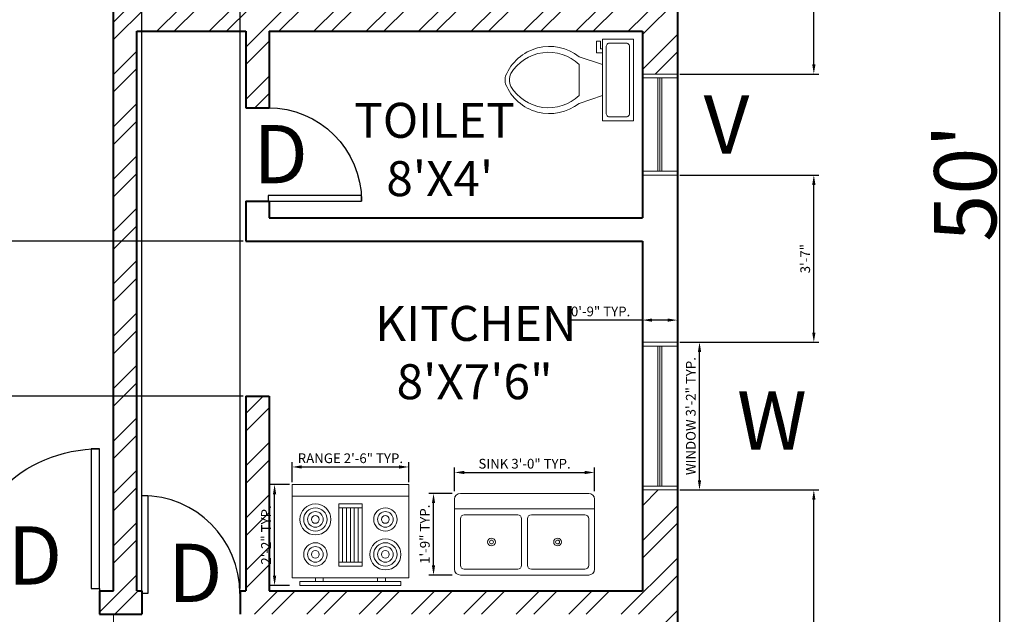
# Model space of a CAD drawing. Units: inches. Extents: x 1143 to 1626, y 7431 to 8140.
# Tile 3 of 4: x 1373 to 1626, y 7656 to 7809. Entities that reach past the tile are written whole.
import ezdxf

# ---------------------------------------------------------------- set-up
doc = ezdxf.new("R2010")
doc.units = ezdxf.units.IN
doc.linetypes.add('ACAD_ISO02W100', pattern=[15, 12, -3])
for name, color, linetype, lineweight in [('A-ANNO-DIMS', 4, 'Continuous', 18), ('A-DOOR', 3, 'Continuous', 25), ('A-FLOR-PRKG', 2, 'ACAD_ISO02W100', 18), ('A-GLAZ', 4, 'Continuous', 18), ('A-WALL', 2, 'Continuous', 40), ('A-WALL-PATT', 7, 'Continuous', 13)]:
    doc.layers.add(name, color=color, linetype=linetype, lineweight=lineweight)
for name, color, linetype, lineweight, true_color in [('A-ANNO-TEXT', 40, 'Continuous', 18, 0xf8d731), ('A-AREA-IDEN', 40, 'Continuous', 25, 0xf8d731), ('A-EQPM', 40, 'Continuous', 18, 0xf8d731), ('A-FLOR-FIXT', 40, 'Continuous', 18, 0xf8d731)]:
    doc.layers.add(name, color=color, linetype=linetype, lineweight=lineweight, true_color=true_color)
doc.styles.get("Standard").update_dxf_attribs({"font": 'arial.ttf'})
doc.dimstyles.new('ISO-25', dxfattribs={"dimtxt": 2.5, "dimasz": 2.5, "dimexe": 1.25, "dimexo": 0.625, "dimtad": 1, "dimdec": 0, "dimlunit": 3, "dimtxsty": 'Standard', "dimcen": 2.5, "dimadec": 0, "dimazin": 0, "dimtfac": 1, "dimtdec": 0, "dimtmove": 0, "dimatfit": 3, "dimfxl": 1, "dimarcsym": 0})

# ---------------------------------------------------------------- blocks, each defined once
blk = doc.blocks.new('*U8')
for p, q in [((0, 0), (0, -100)), ((750, 0), (750, -100))]:
    blk.add_line(p, q)
blk.add_lwpolyline([(0, 0), (0, 750), (43.75, 750), (43.75, 0)], close=True)
blk.add_arc((0, 0), 750, 0, 90)
blk = doc.blocks.new('Range-Oven - 30 in top')
for p, q in [((0, -3), (30, -3)), ((12, -6), (18, -6)), ((13, -20), (13, -6)), ((14, -6), (14, -20)), ((15, -20), (15, -6)), ((16, -6), (16, -20)), ((17, -20), (17, -6)), ((18, -20), (12, -20)), ((6, -24), (6, -25)), ((8, -25), (8, -24)), ((22, -25), (22, -24)), ((24, -24), (24, -25))]:
    blk.add_line(p, q)
for points in [[(0, -24), (0, 0), (30, 0), (30, -24)], [(12, -21), (12, -5), (18, -5), (18, -21)], [(2, -26), (2, -25), (28, -25), (28, -26)]]:
    blk.add_lwpolyline(points, close=True)
for centre, radius in [((6, -9), 4), ((6, -9), 3), ((6, -9), 2), ((24, -9), 3), ((24, -9), 2), ((6, -9), 1), ((24, -9), 1), ((6, -18), 3), ((24, -18), 4), ((24, -18), 3), ((6, -18), 2), ((6, -18), 1), ((24, -18), 2), ((24, -18), 1)]:
    blk.add_circle(centre, radius)
blk = doc.blocks.new('Sink-double - 36 in top')
for p, q in [((-18, -4), (18, -4)), ((-0.75, -18.5), (-0.75, -6.5)), ((0.75, -6.5), (0.75, -18.5))]:
    blk.add_line(p, q)
for points in [[(-16.5, 0), (16.5, 0)], [(-18, -19.5), (-18, -1.5)], [(18, -1.5), (18, -19.5)], [(-16.5, -18.5), (-16.5, -6.5)], [(-15.5, -5.5), (-1.75, -5.5)], [(1.75, -5.5), (15.5, -5.5)], [(16.5, -6.5), (16.5, -18.5)], [(-1.75, -19.5), (-15.5, -19.5)], [(15.5, -19.5), (1.75, -19.5)], [(16.5, -21), (-16.5, -21)]]:
    blk.add_lwpolyline(points)
for centre, radius in [((-8.5, -12.5), 1), ((-8.5, -12.5), 0.5), ((8.5, -12.5), 1), ((8.5, -12.5), 0.5)]:
    blk.add_circle(centre, radius)
for centre, radius, start, end in [((-16.5, -1.5), 1.5, 90, 180), ((16.5, -1.5), 1.5, 0, 90), ((-15.5, -6.5), 1, 90, 180), ((-1.75, -6.5), 1, 0, 90), ((1.75, -6.5), 1, 90, 180), ((15.5, -6.5), 1, 0, 90), ((-16.5, -19.5), 1.5, 180, 270), ((-15.5, -18.5), 1, 180, 270), ((-1.75, -18.5), 1, 270, 0), ((1.75, -18.5), 1, 180, 270), ((15.5, -18.5), 1, 270, 0), ((16.5, -19.5), 1.5, 270, 0)]:
    blk.add_arc(centre, radius, start, end)
blk = doc.blocks.new('Toilet - top')
for p, q in [((9.5, -6), (9.5, -2)), ((-10, -8.5), (-8, -8.5)), ((-10, -9.5), (-10, -8.5)), ((-7, -9.5), (-10, -9.5)), ((-8, -8.5), (-8, -8)), ((-7, -8), (-7, -9.5)), ((-4, -8), (-6, -14)), ((4, -8), (6, -14)), ((4, -14), (-4, -14))]:
    blk.add_line(p, q)
blk.add_lwpolyline([(10.5, -8), (10.5, 0), (-10.5, 0), (-10.5, -8)], close=True)
for points in [[(-9.5, -2), (-9.5, -6)], [(8.5, -1), (-8.5, -1)], [(-8.5, -7), (8.5, -7)]]:
    blk.add_lwpolyline(points)
for centre, radius, start, end in [((-8.62, -1.88), 0.884, 81.8699, 188.1301), ((8.62, -1.88), 0.884, 351.8699, 98.1301), ((-8.62, -6.12), 0.884, 171.8699, 278.1301), ((8.62, -6.12), 0.884, 261.8699, 8.1301), ((3.52, -21.58), 12.17, 141.4691, 247.9714), ((4.2, -21.82), 11.33, 136.3677, 238.9468), ((-3.52, -21.58), 12.17, 292.0284, 38.5307), ((-4.2, -21.82), 11.33, 301.053, 43.6321), ((0, -27.88), 4, 245.7318, 294.2682), ((0, -29), 4, 254.8605, 285.1395)]:
    blk.add_arc(centre, radius, start, end)
blk = doc.blocks.new('*D59')
at = {"layer": 'A-ANNO-DIMS', "color": 0, "lineweight": -2, "transparency": 16777216}
for p, q in [((1542.48, 8067.4), (1625.93, 8067.4)), ((1624.68, 8064.9), (1624.68, 7469.9)), ((1542.48, 7467.4), (1625.93, 7467.4))]:
    blk.add_line(p, q, dxfattribs=at)
at = {"layer": 'A-ANNO-DIMS', "color": 0, "transparency": 16777216}
for points in [[(1624.27, 8064.9), (1625.1, 8064.9), (1624.68, 8067.4)], [(1624.27, 7469.9), (1625.1, 7469.9), (1624.68, 7467.4)]]:
    blk.add_solid(points, dxfattribs=at)
at = {"layer": 'Defpoints', "color": 0, "transparency": 16777216}
for p in [(1541.85, 8067.4), (1541.85, 7467.4), (1624.68, 7467.4)]:
    blk.add_point(p, dxfattribs=at)
at = {"layer": 'A-ANNO-DIMS', "color": 0, "transparency": 16777216, "insert": (1615.89, 7767.4), "char_height": 2.5, "attachment_point": 5, "rotation": 90}
blk.add_mtext("{\\H6.4x;50'}", dxfattribs=at)
blk = doc.blocks.new('WIN-36IN')
for p, q in [((0, 9), (0, 0)), ((1, 9), (1, 0)), ((37, 9), (37, 0)), ((38, 9), (38, 0)), ((1, 5), (37, 5)), ((1, 4.5), (37, 4.5)), ((1, 4), (37, 4))]:
    blk.add_line(p, q)
blk = doc.blocks.new('WIN-24IN')
for p, q in [((0, 9), (0, 0)), ((1, 9), (1, 0)), ((25, 9), (25, 0)), ((26, 9), (26, 0)), ((1, 5), (25, 5)), ((1, 4.5), (25, 4.5)), ((1, 4), (25, 4))]:
    blk.add_line(p, q)
blk = doc.blocks.new('*D62')
at = {"layer": 'A-ANNO-DIMS', "color": 0, "lineweight": -2, "transparency": 16777216}
for p, q in [((1542.48, 7726.4), (1548.8, 7726.4)), ((1547.55, 7690.9), (1547.55, 7723.9)), ((1542.48, 7688.4), (1548.8, 7688.4))]:
    blk.add_line(p, q, dxfattribs=at)
at = {"layer": 'A-ANNO-DIMS', "color": 0, "transparency": 16777216}
for points in [[(1547.13, 7723.9), (1547.97, 7723.9), (1547.55, 7726.4)], [(1547.13, 7690.9), (1547.97, 7690.9), (1547.55, 7688.4)]]:
    blk.add_solid(points, dxfattribs=at)
at = {"layer": 'Defpoints', "color": 0, "transparency": 16777216}
for p in [(1541.85, 7726.4), (1547.55, 7726.4), (1541.85, 7688.4)]:
    blk.add_point(p, dxfattribs=at)
at = {"layer": 'A-ANNO-DIMS', "color": 0, "transparency": 16777216, "insert": (1545.63, 7707.4), "char_height": 2.5, "attachment_point": 5, "rotation": 90}
blk.add_mtext('WINDOW 3\'-2" TYP.', dxfattribs=at)
blk = doc.blocks.new('*D63')
at = {"layer": 'A-ANNO-DIMS', "color": 0, "lineweight": -2, "transparency": 16777216}
for p, q in [((1532.85, 7727.02), (1532.85, 7733.35)), ((1541.85, 7727.02), (1541.85, 7733.35)), ((1532.85, 7732.1), (1513.86, 7732.1)), ((1539.35, 7732.1), (1535.35, 7732.1))]:
    blk.add_line(p, q, dxfattribs=at)
at = {"layer": 'A-ANNO-DIMS', "color": 0, "transparency": 16777216}
for points in [[(1535.35, 7732.51), (1535.35, 7731.68), (1532.85, 7732.1)], [(1539.35, 7732.51), (1539.35, 7731.68), (1541.85, 7732.1)]]:
    blk.add_solid(points, dxfattribs=at)
at = {"layer": 'Defpoints', "color": 0, "transparency": 16777216}
for p in [(1532.85, 7732.1), (1532.85, 7726.4), (1541.85, 7726.4)]:
    blk.add_point(p, dxfattribs=at)
at = {"layer": 'A-ANNO-DIMS', "color": 0, "transparency": 16777216, "insert": (1522.11, 7734), "char_height": 2.5, "attachment_point": 5}
blk.add_mtext('0\'-9" TYP.', dxfattribs=at)
blk = doc.blocks.new('*D76')
at = {"layer": 'A-ANNO-DIMS', "color": 0, "lineweight": -2, "transparency": 16777216}
for p, q in [((1442.77, 7690.44), (1442.77, 7695.56)), ((1472.77, 7690.44), (1472.77, 7695.56)), ((1445.27, 7694.31), (1470.27, 7694.31))]:
    blk.add_line(p, q, dxfattribs=at)
at = {"layer": 'A-ANNO-DIMS', "color": 0, "transparency": 16777216}
for points in [[(1445.27, 7694.73), (1445.27, 7693.89), (1442.77, 7694.31)], [(1470.27, 7694.73), (1470.27, 7693.89), (1472.77, 7694.31)]]:
    blk.add_solid(points, dxfattribs=at)
at = {"layer": 'Defpoints', "color": 0, "transparency": 16777216}
for p in [(1472.77, 7694.31), (1442.77, 7689.81), (1472.77, 7689.81)]:
    blk.add_point(p, dxfattribs=at)
at = {"layer": 'A-ANNO-DIMS', "color": 0, "transparency": 16777216, "insert": (1457.77, 7696.23), "char_height": 2.5, "attachment_point": 5}
blk.add_mtext('RANGE 2\'-6" TYP.', dxfattribs=at)
blk = doc.blocks.new('*D77')
at = {"layer": 'A-ANNO-DIMS', "color": 0, "lineweight": -2, "transparency": 16777216}
for p, q in [((1442.15, 7689.81), (1437.02, 7689.81)), ((1438.27, 7666.31), (1438.27, 7687.31)), ((1442.15, 7663.81), (1437.02, 7663.81))]:
    blk.add_line(p, q, dxfattribs=at)
at = {"layer": 'A-ANNO-DIMS', "color": 0, "transparency": 16777216}
for points in [[(1437.86, 7687.31), (1438.69, 7687.31), (1438.27, 7689.81)], [(1437.86, 7666.31), (1438.69, 7666.31), (1438.27, 7663.81)]]:
    blk.add_solid(points, dxfattribs=at)
at = {"layer": 'Defpoints', "color": 0, "transparency": 16777216}
for p in [(1438.27, 7689.81), (1442.77, 7689.81), (1442.77, 7663.81)]:
    blk.add_point(p, dxfattribs=at)
at = {"layer": 'A-ANNO-DIMS', "color": 0, "transparency": 16777216, "insert": (1436.39, 7676.81), "char_height": 2.5, "attachment_point": 5, "rotation": 90}
blk.add_mtext('2\'-2" TYP.', dxfattribs=at)
blk = doc.blocks.new('*D78')
at = {"layer": 'A-ANNO-DIMS', "color": 0, "lineweight": -2, "transparency": 16777216}
for p, q in [((1484.55, 7688.12), (1484.55, 7694.15)), ((1487.05, 7692.9), (1518.05, 7692.9)), ((1520.55, 7688.12), (1520.55, 7694.15))]:
    blk.add_line(p, q, dxfattribs=at)
at = {"layer": 'A-ANNO-DIMS', "color": 0, "transparency": 16777216}
for points in [[(1487.05, 7693.31), (1487.05, 7692.48), (1484.55, 7692.9)], [(1518.05, 7693.31), (1518.05, 7692.48), (1520.55, 7692.9)]]:
    blk.add_solid(points, dxfattribs=at)
at = {"layer": 'Defpoints', "color": 0, "transparency": 16777216}
for p in [(1520.55, 7692.9), (1484.55, 7687.5), (1520.55, 7687.5)]:
    blk.add_point(p, dxfattribs=at)
at = {"layer": 'A-ANNO-DIMS', "color": 0, "transparency": 16777216, "insert": (1502.55, 7694.82), "char_height": 2.5, "attachment_point": 5}
blk.add_mtext('SINK 3\'-0" TYP.', dxfattribs=at)
blk = doc.blocks.new('*D79')
at = {"layer": 'A-ANNO-DIMS', "color": 0, "lineweight": -2, "transparency": 16777216}
for p, q in [((1483.92, 7687.5), (1477.9, 7687.5)), ((1479.15, 7669), (1479.15, 7685)), ((1483.92, 7666.5), (1477.9, 7666.5))]:
    blk.add_line(p, q, dxfattribs=at)
at = {"layer": 'A-ANNO-DIMS', "color": 0, "transparency": 16777216}
for points in [[(1478.73, 7685), (1479.56, 7685), (1479.15, 7687.5)], [(1478.73, 7669), (1479.56, 7669), (1479.15, 7666.5)]]:
    blk.add_solid(points, dxfattribs=at)
at = {"layer": 'Defpoints', "color": 0, "transparency": 16777216}
for p in [(1479.15, 7687.5), (1484.55, 7687.5), (1484.55, 7666.5)]:
    blk.add_point(p, dxfattribs=at)
at = {"layer": 'A-ANNO-DIMS', "color": 0, "transparency": 16777216, "insert": (1477.24, 7677), "char_height": 2.5, "attachment_point": 5, "rotation": 90}
blk.add_mtext('1\'-9" TYP.', dxfattribs=at)
blk = doc.blocks.new('*D94')
at = {"layer": 'A-ANNO-DIMS', "color": 0, "lineweight": -2, "transparency": 16777216}
for p, q in [((1542.48, 7688.4), (1578.2, 7688.4)), ((1576.95, 7469.9), (1576.95, 7685.9)), ((1542.48, 7467.4), (1578.2, 7467.4))]:
    blk.add_line(p, q, dxfattribs=at)
at = {"layer": 'A-ANNO-DIMS', "color": 0, "transparency": 16777216}
for points in [[(1576.53, 7685.9), (1577.37, 7685.9), (1576.95, 7688.4)], [(1576.53, 7469.9), (1577.37, 7469.9), (1576.95, 7467.4)]]:
    blk.add_solid(points, dxfattribs=at)
at = {"layer": 'Defpoints', "color": 0, "transparency": 16777216}
for p in [(1541.85, 7688.4), (1576.95, 7688.4), (1541.85, 7467.4)]:
    blk.add_point(p, dxfattribs=at)
at = {"layer": 'A-ANNO-DIMS', "color": 0, "transparency": 16777216, "insert": (1575.05, 7577.9), "char_height": 2.5, "attachment_point": 5, "rotation": 90}
blk.add_mtext('18\'-5"', dxfattribs=at)
blk = doc.blocks.new('*D95')
at = {"layer": 'A-ANNO-DIMS', "color": 0, "lineweight": -2, "transparency": 16777216}
for p, q in [((1542.48, 7769.4), (1578.2, 7769.4)), ((1576.95, 7728.9), (1576.95, 7766.9)), ((1542.48, 7726.4), (1578.2, 7726.4))]:
    blk.add_line(p, q, dxfattribs=at)
at = {"layer": 'A-ANNO-DIMS', "color": 0, "transparency": 16777216}
for points in [[(1576.53, 7766.9), (1577.37, 7766.9), (1576.95, 7769.4)], [(1576.53, 7728.9), (1577.37, 7728.9), (1576.95, 7726.4)]]:
    blk.add_solid(points, dxfattribs=at)
at = {"layer": 'Defpoints', "color": 0, "transparency": 16777216}
for p in [(1541.85, 7769.4), (1576.95, 7769.4), (1541.85, 7726.4)]:
    blk.add_point(p, dxfattribs=at)
at = {"layer": 'A-ANNO-DIMS', "color": 0, "transparency": 16777216, "insert": (1575.05, 7747.9), "char_height": 2.5, "attachment_point": 5, "rotation": 90}
blk.add_mtext('3\'-7"', dxfattribs=at)
blk = doc.blocks.new('*D96')
at = {"layer": 'A-ANNO-DIMS', "color": 0, "lineweight": -2, "transparency": 16777216}
for p, q in [((1542.48, 7853.4), (1578.2, 7853.4)), ((1576.95, 7797.9), (1576.95, 7850.9)), ((1542.48, 7795.4), (1578.2, 7795.4))]:
    blk.add_line(p, q, dxfattribs=at)
at = {"layer": 'A-ANNO-DIMS', "color": 0, "transparency": 16777216}
for points in [[(1576.53, 7850.9), (1577.37, 7850.9), (1576.95, 7853.4)], [(1576.53, 7797.9), (1577.37, 7797.9), (1576.95, 7795.4)]]:
    blk.add_solid(points, dxfattribs=at)
at = {"layer": 'Defpoints', "color": 0, "transparency": 16777216}
for p in [(1541.85, 7853.4), (1576.95, 7853.4), (1541.85, 7795.4)]:
    blk.add_point(p, dxfattribs=at)
at = {"layer": 'A-ANNO-DIMS', "color": 0, "transparency": 16777216, "insert": (1575.05, 7824.4), "char_height": 2.5, "attachment_point": 5, "rotation": 90}
blk.add_mtext('4\'-10"', dxfattribs=at)
blk = doc.blocks.new('*D102')
at = {"layer": 'A-ANNO-DIMS', "color": 0, "lineweight": -2, "transparency": 16777216}
for p, q in [((1404.17, 7663.02), (1404.17, 8103.75)), ((1429.38, 7663.02), (1429.38, 8103.75)), ((1406.67, 8102.5), (1426.88, 8102.5))]:
    blk.add_line(p, q, dxfattribs=at)
at = {"layer": 'A-ANNO-DIMS', "color": 0, "transparency": 16777216}
for points in [[(1406.67, 8102.91), (1406.67, 8102.08), (1404.17, 8102.5)], [(1426.88, 8102.91), (1426.88, 8102.08), (1429.38, 8102.5)]]:
    blk.add_solid(points, dxfattribs=at)
at = {"layer": 'Defpoints', "color": 0, "transparency": 16777216}
for p in [(1429.38, 8102.5), (1404.17, 7662.4), (1429.38, 7662.4)]:
    blk.add_point(p, dxfattribs=at)
at = {"layer": 'A-ANNO-DIMS', "color": 0, "transparency": 16777216, "insert": (1416.78, 8104.38), "char_height": 2.5, "attachment_point": 5}
blk.add_mtext('2\'-1"', dxfattribs=at)
blk = doc.blocks.new('*D103')
at = {"layer": 'A-ANNO-DIMS', "color": 0, "lineweight": -2, "transparency": 16777216}
for p, q in [((1430.23, 7752.4), (1145.5, 7752.4)), ((1146.75, 7715.06), (1146.75, 7749.9)), ((1430.23, 7712.56), (1145.5, 7712.56))]:
    blk.add_line(p, q, dxfattribs=at)
at = {"layer": 'A-ANNO-DIMS', "color": 0, "transparency": 16777216}
for points in [[(1146.33, 7749.9), (1147.17, 7749.9), (1146.75, 7752.4)], [(1146.33, 7715.06), (1147.17, 7715.06), (1146.75, 7712.56)]]:
    blk.add_solid(points, dxfattribs=at)
at = {"layer": 'Defpoints', "color": 0, "transparency": 16777216}
for p in [(1146.75, 7752.4), (1430.85, 7752.4), (1430.85, 7712.56)]:
    blk.add_point(p, dxfattribs=at)
at = {"layer": 'A-ANNO-DIMS', "color": 0, "transparency": 16777216, "insert": (1144.85, 7732.48), "char_height": 2.5, "attachment_point": 5, "rotation": 90}
blk.add_mtext('3\'-4"', dxfattribs=at)

msp = doc.modelspace()

# ---------------------------------------------------------------- hatches: boundary and pattern name
at = {"layer": 'A-WALL-PATT'}
h = msp.add_hatch(dxfattribs=at)
h.set_pattern_fill('ANSI32', color=256)
h.paths.add_polyline_path([(1240.85, 8067.4), (1181.85, 8067.4), (1181.85, 8017.4), (1190.85, 8017.4), (1190.85, 8058.4), (1240.85, 8058.4)])
h.paths.add_polyline_path([(1541.85, 8067.4), (1486.85, 8067.4), (1486.85, 8058.4), (1532.85, 8058.4), (1532.85, 8017.4), (1541.85, 8017.4)], flags=17)
h.paths.add_polyline_path([(1352.85, 8067.4), (1278.85, 8067.4), (1278.85, 8058.4), (1328.85, 8058.4), (1328.85, 7938.4), (1319.96, 7938.4), (1319.96, 7932.4), (1334.85, 7932.4), (1334.85, 7956.4), (1338.11, 7956.4), (1338.11, 7962.4), (1334.85, 7962.4), (1334.85, 8010.4), (1396.85, 8010.4), (1396.85, 7962.4), (1386.11, 7962.4), (1386.11, 7956.4), (1396.85, 7956.4), (1396.85, 7662.4), (1393.24, 7662.4), (1393.24, 7656.4), (1404.17, 7656.4), (1404.17, 7662.4), (1402.85, 7662.4), (1402.85, 7806.4), (1430.85, 7806.4), (1430.85, 7786.73), (1436.85, 7786.73), (1436.85, 7806.4), (1532.85, 7806.4), (1532.85, 7795.4), (1541.85, 7795.4), (1541.85, 7853.4), (1532.85, 7853.4), (1532.85, 7812.4), (1402.85, 7812.4), (1402.85, 7932.4), (1419.12, 7932.4), (1419.12, 7938.4), (1402.85, 7938.4), (1402.85, 8058.4), (1448.85, 8058.4), (1448.85, 8067.4), (1378.85, 8067.4), (1378.85, 8058.4), (1396.85, 8058.4), (1396.85, 8016.4), (1334.85, 8016.4), (1334.85, 8058.4), (1352.85, 8058.4)])
h.paths.add_polyline_path([(1283.96, 7938.4), (1190.85, 7938.4), (1190.85, 7979.4), (1181.85, 7979.4), (1181.85, 7903.4), (1190.85, 7903.4), (1190.85, 7932.4), (1238.85, 7932.4), (1238.85, 7848.4), (1234.31, 7848.4), (1234.31, 7842.4), (1244.85, 7842.4), (1244.85, 7932.4), (1283.96, 7932.4)])
h.paths.add_polyline_path([(1541.85, 7979.4), (1532.85, 7979.4), (1532.85, 7938.4), (1455.12, 7938.4), (1455.12, 7932.4), (1532.85, 7932.4), (1532.85, 7891.4), (1541.85, 7891.4)], flags=17)
h.paths.add_polyline_path([(1210.81, 7716.4), (1190.85, 7716.4), (1190.85, 7745.4), (1181.85, 7745.4), (1181.85, 7663.4), (1190.85, 7663.4), (1190.85, 7710.4), (1210.81, 7710.4)])
h.paths.add_polyline_path([(1232.89, 7871.85), (1232.89, 7871.89), (1234.29, 7871.89), (1234.29, 7847.89), (1232.89, 7847.89), (1232.89, 7871.85, 0.385662), (1210.31, 7848.85), (1210.31, 7842.4), (1190.85, 7842.4), (1190.85, 7806.4), (1244.85, 7806.4), (1244.85, 7716.4), (1325.66, 7716.4), (1334.85, 7716.4), (1334.85, 7706.63), (1328.13, 7706.63), (1328.13, 7704.53), (1292.13, 7704.53), (1292.13, 7706.63), (1328.85, 7706.63), (1328.85, 7710.4), (1325.66, 7710.4), (1234.81, 7710.4), (1234.81, 7716.6), (1233.41, 7716.6), (1233.41, 7740.6), (1234.81, 7740.6), (1234.81, 7716.4), (1238.85, 7716.4), (1238.85, 7800.4), (1190.85, 7800.4), (1190.85, 7770.4), (1186.85, 7770.4), (1186.85, 7746.4), (1185.85, 7746.4), (1185.85, 7770.4), (1181.85, 7770.4), (1181.85, 7878.4), (1190.85, 7878.4), (1190.85, 7848.4), (1210.3, 7848.4, -0.391105)])
h.paths.add_polyline_path([(1541.85, 7688.4), (1532.85, 7688.4), (1532.85, 7662.4), (1436.85, 7662.4), (1436.85, 7712.56), (1430.85, 7712.56), (1430.85, 7662.4), (1429.38, 7656.4), (1532.85, 7656.4), (1532.85, 7467.4), (1541.85, 7467.4)])
h.paths.add_polyline_path([(1334.85, 7656.4), (1357.24, 7656.4), (1357.24, 7662.4), (1334.85, 7662.4), (1334.85, 7670.63), (1328.85, 7670.63), (1328.85, 7618.14), (1334.85, 7618.14)])
h.paths.add_polyline_path([(1190.85, 7572.4), (1334.85, 7572.4), (1334.85, 7582.14), (1328.85, 7582.14), (1328.85, 7578.4), (1190.85, 7578.4), (1190.85, 7625.4), (1181.85, 7625.4), (1181.85, 7467.4), (1324.72, 7467.4), (1324.72, 7476.4), (1190.85, 7476.4)])

# ---------------------------------------------------------------- linework, layer by layer
at = {"layer": 'A-FLOR-PRKG'}
msp.add_line((1396.85, 7656.4), (1396.85, 7476.4), dxfattribs=at)
at = {"layer": 'A-WALL'}
for p, q in [((1541.85, 8067.4), (1541.85, 7467.4)), ((1396.85, 7662.4), (1396.85, 7956.4)), ((1402.85, 7806.4), (1430.85, 7806.4)), ((1402.85, 7662.4), (1402.85, 7806.4)), ((1430.85, 7806.4), (1430.85, 7786.73)), ((1436.85, 7806.4), (1436.85, 7786.73)), ((1436.85, 7806.4), (1532.85, 7806.4)), ((1532.85, 7806.4), (1532.85, 7758.4)), ((1430.85, 7786.73), (1436.85, 7786.73)), ((1430.85, 7762.73), (1436.85, 7762.73)), ((1430.85, 7762.73), (1430.85, 7752.4)), ((1436.85, 7762.73), (1436.85, 7758.4)), ((1436.85, 7758.4), (1532.85, 7758.4)), ((1430.85, 7752.4), (1532.85, 7752.4)), ((1532.85, 7752.4), (1532.85, 7662.4)), ((1430.85, 7712.56), (1436.85, 7712.56)), ((1430.85, 7712.56), (1430.85, 7662.4)), ((1436.85, 7712.56), (1436.85, 7662.4)), ((1393.24, 7662.4), (1393.24, 7656.4)), ((1393.24, 7662.4), (1396.85, 7662.4)), ((1402.85, 7662.4), (1404.17, 7662.4)), ((1404.17, 7662.4), (1404.17, 7656.4)), ((1429.38, 7662.4), (1429.38, 7656.4)), ((1429.38, 7662.4), (1430.85, 7662.4)), ((1436.85, 7662.4), (1532.85, 7662.4)), ((1393.24, 7656.4), (1404.17, 7656.4))]:
    msp.add_line(p, q, dxfattribs=at)

# ---------------------------------------------------------------- block references
at = {"layer": 'A-DOOR', "xscale": -0.0320363486803998, "yscale": 0.0320363486803998, "zscale": 0.0320363486803998, "rotation": 270}
msp.add_blockref('*U8', (1436.6, 7762.73), dxfattribs=at)
at = {"layer": 'A-DOOR'}
for p, xscale, yscale, zscale in [((1393.24, 7663), -0.0480000000000001, 0.0480000000000001, 0.0480000000000001), ((1404.17, 7661.75), 0.0336011074731409, 0.0336011074731409, 0.0336011074731409)]:
    msp.add_blockref('*U8', p, dxfattribs=dict(at, xscale=xscale, yscale=yscale, zscale=zscale))
at = {"layer": 'A-EQPM'}
msp.add_blockref('Range-Oven - 30 in top', (1442.77, 7689.81), dxfattribs=at)
at = {"layer": 'A-FLOR-FIXT', "rotation": 270}
msp.add_blockref('Toilet - top', (1530.56, 7793.87), dxfattribs=at)
at = {"layer": 'A-FLOR-FIXT'}
msp.add_blockref('Sink-double - 36 in top', (1502.55, 7687.5), dxfattribs=at)
at = {"layer": 'A-GLAZ'}
for name, p, rotation in [('WIN-24IN', (1532.85, 7795.4), 269.9999999999985), ('WIN-36IN', (1541.85, 7688.4), 89.99999999999628)]:
    msp.add_blockref(name, p, dxfattribs=dict(at, rotation=rotation))

# ---------------------------------------------------------------- texts
at = {"layer": 'A-ANNO-TEXT', "char_height": 15, "attachment_point": 1}
for s, insert in [('{V}', (1548.6, 7789.96)), ('{D}', (1432.77, 7782.3)), ('{W}', (1557.19, 7713.76)), ('{D}', (1369.59, 7679.04)), ('{D}', (1410.82, 7674.56))]:
    msp.add_mtext_dynamic_manual_height_columns(s, width=1087.9578, gutter_width=12.5, heights=[0], dxfattribs=dict(at, insert=insert))
at = {"layer": 'A-AREA-IDEN', "char_height": 9, "attachment_point": 1}
for s, insert in [("{       TOILET\\P          8'X4'}", (1439.5, 7788)), ('{     KITCHEN\\P       8\'X7\'6"}', (1450.4, 7735.75))]:
    msp.add_mtext_dynamic_manual_height_columns(s, width=1087.9578, gutter_width=12.5, heights=[0], dxfattribs=dict(at, insert=insert))

# ---------------------------------------------------------------- dimensions: what is measured, and where the dimension line sits
at = {"layer": 'A-ANNO-DIMS'}
dim = msp.add_linear_dim(base=(1429.38, 8102.5), p1=(1404.17, 7662.4), p2=(1429.38, 7662.4), dimstyle='ISO-25', override={"dimdec": 1, "dimlfac": 1, "dimrnd": 0, "dimzin": 1, "dimdsep": 46, "dimlunit": 4, "dimfrac": 2}, dxfattribs=at)
dim.commit()
dim.dimension.update_dxf_attribs({"geometry": '*D102', "text_midpoint": (1416.78, 8104.38)})
for base, p1, p2, angle, text, override, picture, middle in [((1624.68, 7467.4), (1541.85, 8067.4), (1541.85, 7467.4), 90, '{\\H6.4x;<>}', {"dimclrd": 0, "dimclre": 0, "dimclrt": 0}, '*D59', (1615.89, 7767.4)), ((1532.85, 7732.1), (1541.85, 7726.4), (1532.85, 7726.4), 180, '<> TYP.', {"dimdec": 1, "dimlfac": 1, "dimrnd": 0, "dimzin": 1, "dimdsep": 46, "dimlunit": 4, "dimfrac": 2}, '*D63', (1522.11, 7734)), ((1547.55, 7726.4), (1541.85, 7688.4), (1541.85, 7726.4), 90, 'WINDOW <> TYP.', {"dimdec": 1, "dimlfac": 1, "dimrnd": 0, "dimzin": 1, "dimdsep": 46, "dimlunit": 4, "dimfrac": 2}, '*D62', (1545.63, 7707.4)), ((1438.27, 7689.81), (1442.77, 7663.81), (1442.77, 7689.81), 90, '<> TYP.', {"dimdec": 1, "dimlfac": 1, "dimrnd": 0, "dimzin": 1, "dimdsep": 46, "dimlunit": 4, "dimfrac": 2}, '*D77', (1436.39, 7676.81)), ((1479.15, 7687.5), (1484.55, 7666.5), (1484.55, 7687.5), 90, '<> TYP.', {"dimdec": 1, "dimlfac": 1, "dimrnd": 0, "dimzin": 1, "dimdsep": 46, "dimlunit": 4, "dimfrac": 2}, '*D79', (1477.24, 7677))]:
    dim = msp.add_linear_dim(base=base, p1=p1, p2=p2, angle=angle, text=text, dimstyle='ISO-25', override=override, dxfattribs=at)
    dim.commit()
    dim.dimension.update_dxf_attribs({"geometry": picture, "text_midpoint": middle})
for base, p1, p2, picture, middle in [((1576.95, 7853.4), (1541.85, 7795.4), (1541.85, 7853.4), '*D96', (1575.05, 7824.4)), ((1576.95, 7769.4), (1541.85, 7726.4), (1541.85, 7769.4), '*D95', (1575.05, 7747.9)), ((1146.75, 7752.4), (1430.85, 7712.56), (1430.85, 7752.4), '*D103', (1144.85, 7732.48)), ((1576.95, 7688.4), (1541.85, 7467.4), (1541.85, 7688.4), '*D94', (1575.05, 7577.9))]:
    dim = msp.add_linear_dim(base=base, p1=p1, p2=p2, angle=90, dimstyle='ISO-25', override={"dimdec": 1, "dimlfac": 1, "dimrnd": 0, "dimzin": 1, "dimdsep": 46, "dimlunit": 4, "dimfrac": 2}, dxfattribs=at)
    dim.commit()
    dim.dimension.update_dxf_attribs({"geometry": picture, "text_midpoint": middle})
for base, p1, p2, text, picture, middle in [((1472.77, 7694.31), (1442.77, 7689.81), (1472.77, 7689.81), 'RANGE <> TYP.', '*D76', (1457.77, 7696.23)), ((1520.55, 7692.9), (1484.55, 7687.5), (1520.55, 7687.5), 'SINK <> TYP.', '*D78', (1502.55, 7694.82))]:
    dim = msp.add_linear_dim(base=base, p1=p1, p2=p2, text=text, dimstyle='ISO-25', override={"dimdec": 1, "dimlfac": 1, "dimrnd": 0, "dimzin": 1, "dimdsep": 46, "dimlunit": 4, "dimfrac": 2}, dxfattribs=at)
    dim.commit()
    dim.dimension.update_dxf_attribs({"geometry": picture, "text_midpoint": middle})

doc.saveas('drawing.dxf')
